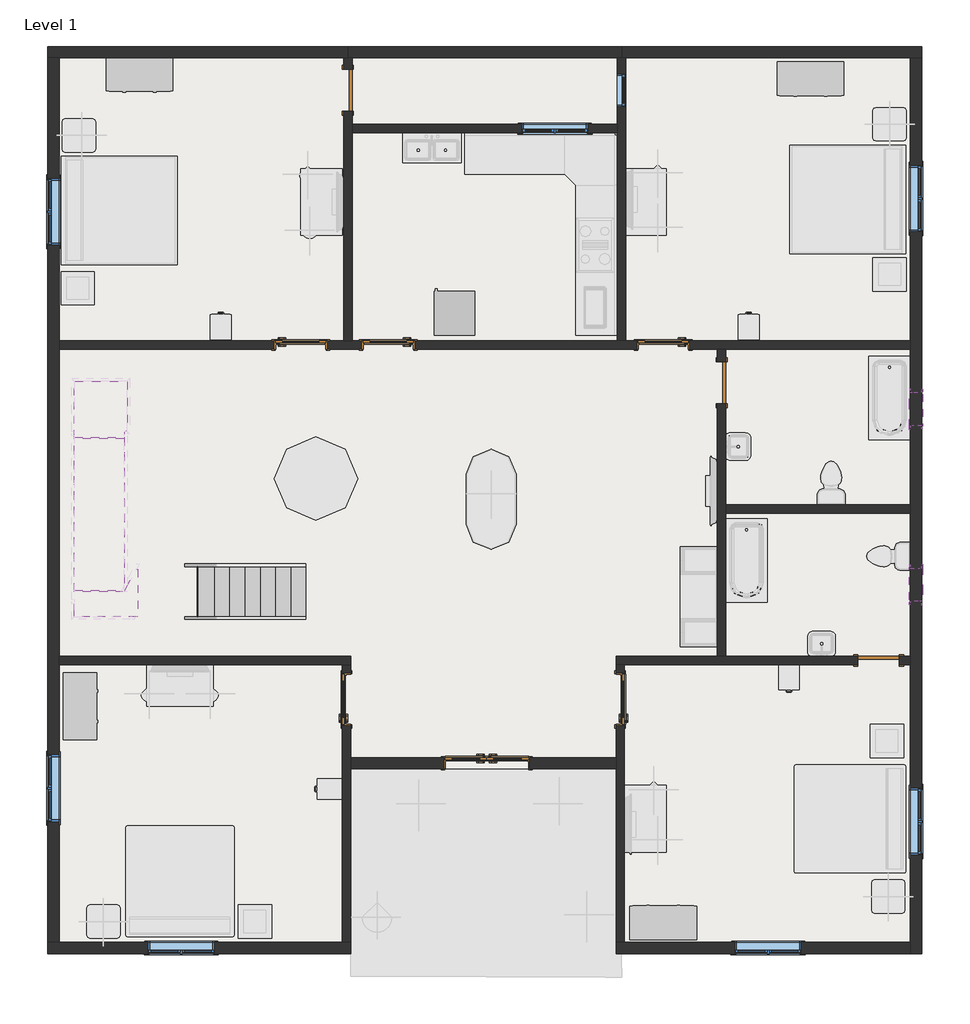
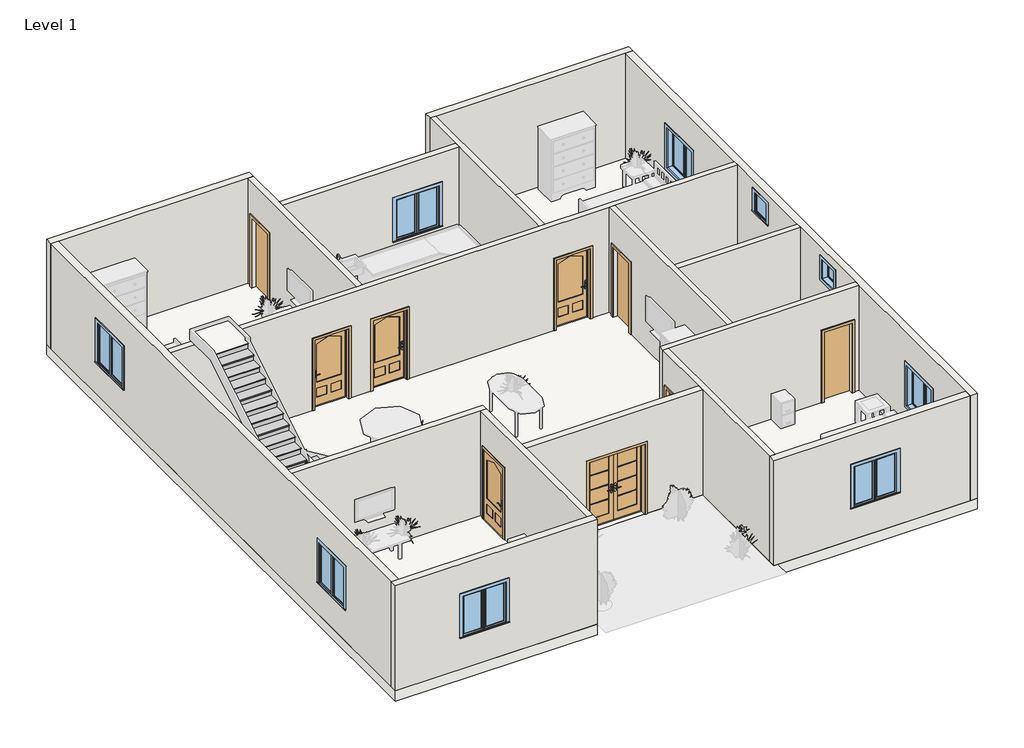
# One storey, part 1 of 2: 18 walls, 10 windows, 9 doors, 3 slabs, 2 stair flights.
"""IFC4 building model written with IfcOpenShell, lengths in millimetres."""

from ifc_helpers import new_model, si_unit, frame, origin, origin_with_axes, place, context, project, spatial, polyline, outline, extrude, faceted_brep, transform, mapped, element, save
from components import door_5d363d20, door_808aeb8e, door_b03bd389, door_059fdd7e, door_255cab33, non_monolithic_landing_7e22f3b9, non_monolithic_landing_d7f15ac0, stair_flight_13c2be00, stair_flight_cee2f43a, window_0862ab64, window_be30da88, window_aff1bc2a, window_e41d21a6

model = new_model("IFC4")

# Units and contexts
model_context = context("Model", 3, world=origin())
ifc_project = project(units=[si_unit("LENGTHUNIT", "METRE", prefix="MILLI")], contexts=[model_context])

# Site, building, storey
site = spatial("IfcSite", under=ifc_project)
building = spatial("IfcBuilding", under=site)
storey = spatial("IfcBuildingStorey", under=building, Name="Level 1", Elevation=0.0)

# Doors
placement = place(None, origin())
door_shape = door_5d363d20(model_context)
element("IfcDoor", 1, ObjectType="36\" x 80\"", at=placement, inside=storey, context=model_context, shape_type="MappedRepresentation", body=[
    mapped(door_shape, transform((-10796.38283, 9355.0370171, 0.0), x_axis=(-1.0, 0.0, 0.0), y_axis=(0.0, -1.0, 0.0), z_axis=(0.0, 0.0, 1.0))),
])
element("IfcDoor", 2, ObjectType="36\" x 80\"", at=placement, inside=storey, context=model_context, shape_type="MappedRepresentation", body=[
    mapped(door_shape, transform((-9961.35783, 2874.8620171, 0.0), x_axis=(0.0, -1.0, 0.0), y_axis=(1.0, 0.0, 0.0), z_axis=(0.0, 0.0, 1.0))),
])
door_2_shape = door_808aeb8e(model_context)
element("IfcDoor", 3, ObjectType="36\" x 80\"", at=placement, inside=storey, context=model_context, shape_type="MappedRepresentation", body=[
    mapped(door_2_shape, transform((-9196.18283, 9355.0370171, 0.0), x_axis=(1.0, 0.0, 0.0), y_axis=(0.0, 1.0, 0.0), z_axis=(0.0, 0.0, 1.0))),
])
element("IfcDoor", 4, ObjectType="36\" x 80\"", at=placement, inside=storey, context=model_context, shape_type="MappedRepresentation", body=[
    mapped(door_2_shape, transform((-4166.98283, 9355.0370171, 0.0), x_axis=(1.0, 0.0, 0.0), y_axis=(0.0, 1.0, 0.0), z_axis=(0.0, 0.0, 1.0))),
])
element("IfcDoor", 5, ObjectType="36\" x 80\"", at=placement, inside=storey, context=model_context, shape_type="MappedRepresentation", body=[
    mapped(door_2_shape, transform((-4951.20783, 2874.8620171, 0.0), x_axis=(0.0, -1.0, 0.0), y_axis=(1.0, 0.0, 0.0), z_axis=(0.0, 0.0, 1.0))),
])
door_3_shape = door_b03bd389(model_context)
element("IfcDoor", 6, ObjectType="Door-Exterior-Double-Full Glass-Wood_Clad : 60\" x 80\"", at=placement, inside=storey, context=model_context, shape_type="MappedRepresentation", body=[
    mapped(door_3_shape, transform((-7392.78283, 1709.6370171, 0.0), x_axis=(1.0, 0.0, 0.0), y_axis=(0.0, 1.0, 0.0), z_axis=(0.0, 0.0, 1.0))),
])
door_4_shape = door_059fdd7e(model_context)
element("IfcDoor", 7, ObjectType="Single-Flush : 30\" x 80\"", at=placement, inside=storey, context=model_context, shape_type="MappedRepresentation", body=[
    mapped(door_4_shape, transform((-229.98283, 3586.0620171, 0.0), x_axis=(1.0, 0.0, 0.0), y_axis=(0.0, 1.0, 0.0), z_axis=(0.0, 0.0, 1.0))),
])
element("IfcDoor", 8, ObjectType="Single-Flush : 30\" x 80\"", at=placement, inside=storey, context=model_context, shape_type="MappedRepresentation", body=[
    mapped(door_4_shape, transform((-9932.78283, 14012.7620171, 0.0), x_axis=(0.0, -1.0, 0.0), y_axis=(1.0, 0.0, 0.0), z_axis=(0.0, 0.0, 1.0))),
])
door_5_shape = door_255cab33(model_context)
element("IfcDoor", 9, ObjectType="Single-Flush : 30\" x 80\"", at=placement, inside=storey, context=model_context, shape_type="MappedRepresentation", body=[
    mapped(door_5_shape, transform((-3100.18283, 8666.0620171, 0.0), x_axis=(0.0, 1.0, 0.0), y_axis=(-1.0, 0.0, 0.0), z_axis=(0.0, 0.0, 1.0))),
])

# Slabs
element("IfcSlab", 10, ObjectType="Generic - 12\"", at=placement, inside=storey, context=model_context, shape_type="SweptSolid", body=[
    extrude(outline(polyline([(557.41717, 14812.8620171), (557.41717, -1773.3379829), (-5030.58283, -1773.3379829), (-5030.58283, 1604.8620171), (-9881.98283, 1604.8620171), (-9881.98283, -1773.3379829), (-15419.18283, -1773.3379829), (-15419.18283, 14812.8620171), (557.41717, 14812.8620171)])), frame((0.0, 0.0, -304.8), z_axis=(0.0, 0.0, 1.0), x_axis=(1.0, 0.0, 0.0)), (0.0, 0.0, 1.0), 304.8),
])
non_monolithic_landing_shape = non_monolithic_landing_7e22f3b9(model_context)
element("IfcSlab", 11, ObjectType="Non-Monolithic Landing", at=placement, inside=storey, context=model_context, shape_type="MappedRepresentation", body=[
    mapped(non_monolithic_landing_shape, transform((0.0, 0.0, 0.0), x_axis=(1.0, 0.0, 0.0), y_axis=(0.0, 1.0, 0.0), z_axis=(0.0, 0.0, 1.0))),
])
non_monolithic_landing_2_shape = non_monolithic_landing_d7f15ac0(model_context)
element("IfcSlab", 12, ObjectType="Non-Monolithic Landing", at=placement, inside=storey, context=model_context, shape_type="MappedRepresentation", body=[
    mapped(non_monolithic_landing_2_shape, transform((0.0, 0.0, 0.0), x_axis=(1.0, 0.0, 0.0), y_axis=(0.0, 1.0, 0.0), z_axis=(0.0, 0.0, 1.0))),
])

# Stair flights
stair_flight_shape = stair_flight_13c2be00(model_context)
element("IfcStairFlight", 13, ObjectType="2\" Tread 1\" Nosing 1/4\" Riser", at=placement, inside=storey, context=model_context, shape_type="MappedRepresentation", body=[
    mapped(stair_flight_shape, transform((0.0, 0.0, 0.0), x_axis=(1.0, 0.0, 0.0), y_axis=(0.0, 1.0, 0.0), z_axis=(0.0, 0.0, 1.0))),
])
stair_flight_2_shape = stair_flight_cee2f43a(model_context)
element("IfcStairFlight", 14, ObjectType="2\" Tread 1\" Nosing 1/4\" Riser", at=placement, inside=storey, context=model_context, shape_type="MappedRepresentation", body=[
    mapped(stair_flight_2_shape, transform((0.0, 0.0, 0.0), x_axis=(1.0, 0.0, 0.0), y_axis=(0.0, 1.0, 0.0), z_axis=(0.0, 0.0, 1.0))),
])

# Walls
element("IfcWall", 15, ObjectType="Generic - 8\"", at=placement, inside=storey, context=model_context, shape_type="Brep", body=[
    faceted_brep([(-15419.18283, 14609.6620171, 0.0), (-15215.98283, 14609.6620171, 0.0), (-10008.98283, 14609.6620171, 0.0), (-9932.78283, 14609.6620171, 0.0), (-9932.78283, 14609.6620171, 1828.8), (-9856.58283, 14609.6620171, 1828.8), (-9856.58283, 14609.6620171, 3048.0), (-10008.98283, 14609.6620171, 3048.0), (-15215.98283, 14609.6620171, 3048.0), (-15419.18283, 14609.6620171, 3048.0), (-15419.18283, 14812.8620171, 0.0), (-15419.18283, 14812.8620171, 3048.0), (-9856.58283, 14812.8620171, 3048.0), (-9856.58283, 14812.8620171, 1828.8), (-9932.78283, 14812.8620171, 1828.8), (-9932.78283, 14812.8620171, 0.0)], [[[0, 1, 2, 3, 4, 5, 6, 7, 8, 9]], [[10, 11, 12, 13, 14, 15]], [[3, 2, 1, 0, 10, 15]], [[0, 9, 11, 10]], [[4, 3, 15, 14]], [[13, 5, 4, 14]], [[6, 5, 13, 12]], [[9, 8, 7, 6, 12, 11]]]),
])
element("IfcWall", 16, ObjectType="Generic - 8\"", at=placement, inside=storey, context=model_context, shape_type="Brep", body=[
    faceted_brep([(354.21717, 14609.6620171, 0.0), (354.21717, 9428.0620171, 0.0), (354.21717, 9275.6620171, 0.0), (354.21717, 6430.8620171, 0.0), (354.21717, 6278.4620171, 0.0), (354.21717, 3662.2620171, 0.0), (354.21717, 3509.8620171, 0.0), (354.21717, -1570.1379829, 0.0), (354.21717, -1773.3379829, 0.0), (354.21717, -1773.3379829, 3048.0), (354.21717, -1570.1379829, 3048.0), (354.21717, 3509.8620171, 3048.0), (354.21717, 3662.2620171, 3048.0), (354.21717, 6278.4620171, 3048.0), (354.21717, 6430.8620171, 3048.0), (354.21717, 9275.6620171, 3048.0), (354.21717, 9428.0620171, 3048.0), (354.21717, 14609.6620171, 3048.0), (354.21717, 11421.9620171, 2133.6), (354.21717, 11421.9620171, 914.4), (354.21717, 12641.1620171, 914.4), (354.21717, 12641.1620171, 2133.6), (354.21717, 30.0620171, 2133.6), (354.21717, 30.0620171, 914.4), (354.21717, 1249.2620171, 914.4), (354.21717, 1249.2620171, 2133.6), (354.21717, 4665.5620171, 2768.6), (354.21717, 4665.5620171, 2159.0), (354.21717, 5275.1620171, 2159.0), (354.21717, 5275.1620171, 2768.6), (354.21717, 8488.2620171, 2768.6), (354.21717, 7878.6620171, 2768.6), (354.21717, 7878.6620171, 2159.0), (354.21717, 8488.2620171, 2159.0), (557.41717, 14609.6620171, 0.0), (557.41717, 14609.6620171, 3048.0), (557.41717, -1773.3379829, 3048.0), (557.41717, -1773.3379829, 0.0), (557.41717, 11421.9620171, 2133.6), (557.41717, 12641.1620171, 2133.6), (557.41717, 12641.1620171, 914.4), (557.41717, 11421.9620171, 914.4), (557.41717, 30.0620171, 2133.6), (557.41717, 1249.2620171, 2133.6), (557.41717, 1249.2620171, 914.4), (557.41717, 30.0620171, 914.4), (557.41717, 4665.5620171, 2768.6), (557.41717, 5275.1620171, 2768.6), (557.41717, 5275.1620171, 2159.0), (557.41717, 4665.5620171, 2159.0), (557.41717, 8488.2620171, 2768.6), (557.41717, 8488.2620171, 2159.0), (557.41717, 7878.6620171, 2159.0), (557.41717, 7878.6620171, 2768.6)], [[[0, 1, 2, 3, 4, 5, 6, 7, 8, 9, 10, 11, 12, 13, 14, 15, 16, 17], [18, 19, 20, 21], [22, 23, 24, 25], [26, 27, 28, 29], [30, 31, 32, 33]], [[34, 35, 36, 37], [38, 39, 40, 41], [42, 43, 44, 45], [46, 47, 48, 49], [50, 51, 52, 53]], [[8, 7, 6, 5, 4, 3, 2, 1, 0, 34, 37]], [[0, 17, 35, 34]], [[9, 8, 37, 36]], [[19, 18, 38, 41]], [[20, 19, 41, 40]], [[21, 20, 40, 39]], [[18, 21, 39, 38]], [[23, 22, 42, 45]], [[24, 23, 45, 44]], [[25, 24, 44, 43]], [[22, 25, 43, 42]], [[27, 26, 46, 49]], [[28, 27, 49, 48]], [[29, 28, 48, 47]], [[26, 29, 47, 46]], [[51, 50, 30, 33]], [[52, 51, 33, 32]], [[53, 52, 32, 31]], [[50, 53, 31, 30]], [[17, 16, 15, 14, 13, 12, 11, 10, 9, 36, 35]]]),
])
element("IfcWall", 17, ObjectType="Generic - 8\"", at=placement, inside=storey, context=model_context, shape_type="Brep", body=[
    faceted_brep([(354.21717, -1570.1379829, 0.0), (-4878.18283, -1570.1379829, 0.0), (-5030.58283, -1570.1379829, 0.0), (-5030.58283, -1570.1379829, 3048.0), (-4878.18283, -1570.1379829, 3048.0), (354.21717, -1570.1379829, 3048.0), (-2858.88283, -1570.1379829, 2133.6), (-2858.88283, -1570.1379829, 914.4), (-1639.68283, -1570.1379829, 914.4), (-1639.68283, -1570.1379829, 2133.6), (354.21717, -1773.3379829, 0.0), (354.21717, -1773.3379829, 3048.0), (-5030.58283, -1773.3379829, 3048.0), (-5030.58283, -1773.3379829, 0.0), (-2858.88283, -1773.3379829, 2133.6), (-1639.68283, -1773.3379829, 2133.6), (-1639.68283, -1773.3379829, 914.4), (-2858.88283, -1773.3379829, 914.4)], [[[0, 1, 2, 3, 4, 5], [6, 7, 8, 9]], [[10, 11, 12, 13], [14, 15, 16, 17]], [[2, 1, 0, 10, 13]], [[0, 5, 11, 10]], [[3, 2, 13, 12]], [[7, 6, 14, 17]], [[8, 7, 17, 16]], [[9, 8, 16, 15]], [[6, 9, 15, 14]], [[5, 4, 3, 12, 11]]]),
])
element("IfcWall", 18, ObjectType="Generic - 8\"", at=placement, inside=storey, context=model_context, shape_type="Brep", body=[
    faceted_brep([(-15215.98283, -1570.1379829, 0.0), (-15215.98283, 3509.8620171, 0.0), (-15215.98283, 3662.2620171, 0.0), (-15215.98283, 9275.6620171, 0.0), (-15215.98283, 9428.0620171, 0.0), (-15215.98283, 14609.6620171, 0.0), (-15215.98283, 14609.6620171, 3048.0), (-15215.98283, 9428.0620171, 3048.0), (-15215.98283, 9275.6620171, 3048.0), (-15215.98283, 3662.2620171, 3048.0), (-15215.98283, 3509.8620171, 3048.0), (-15215.98283, -1570.1379829, 3048.0), (-15215.98283, 12399.8620171, 2133.6), (-15215.98283, 12399.8620171, 914.4), (-15215.98283, 11180.6620171, 914.4), (-15215.98283, 11180.6620171, 2133.6), (-15215.98283, 1858.8620171, 2133.6), (-15215.98283, 1858.8620171, 914.4), (-15215.98283, 639.6620171, 914.4), (-15215.98283, 639.6620171, 2133.6), (-15419.18283, -1570.1379829, 0.0), (-15419.18283, -1570.1379829, 3048.0), (-15419.18283, 14609.6620171, 3048.0), (-15419.18283, 14609.6620171, 0.0), (-15419.18283, 12399.8620171, 2133.6), (-15419.18283, 11180.6620171, 2133.6), (-15419.18283, 11180.6620171, 914.4), (-15419.18283, 12399.8620171, 914.4), (-15419.18283, 1858.8620171, 2133.6), (-15419.18283, 639.6620171, 2133.6), (-15419.18283, 639.6620171, 914.4), (-15419.18283, 1858.8620171, 914.4)], [[[0, 1, 2, 3, 4, 5, 6, 7, 8, 9, 10, 11], [12, 13, 14, 15], [16, 17, 18, 19]], [[20, 21, 22, 23], [24, 25, 26, 27], [28, 29, 30, 31]], [[5, 4, 3, 2, 1, 0, 20, 23]], [[6, 5, 23, 22]], [[0, 11, 21, 20]], [[13, 12, 24, 27]], [[14, 13, 27, 26]], [[15, 14, 26, 25]], [[12, 15, 25, 24]], [[17, 16, 28, 31]], [[18, 17, 31, 30]], [[19, 18, 30, 29]], [[16, 19, 29, 28]], [[11, 10, 9, 8, 7, 6, 22, 21]]]),
])
element("IfcWall", 19, ObjectType="Generic - 8\"", at=placement, inside=storey, context=model_context, shape_type="SweptSolid", body=[
    extrude(outline(polyline([(3048.0, -9881.98283), (0.0, -9881.98283), (0.0, -8180.18283), (2057.4, -8180.18283), (2057.4, -6605.38283), (0.0, -6605.38283), (0.0, -5030.58283), (3048.0, -5030.58283), (3048.0, -9881.98283)])), frame((0.0, 1604.8620171, 0.0), z_axis=(0.0, 1.0, 0.0), x_axis=(0.0, 0.0, 1.0)), (0.0, 0.0, 1.0), 203.2),
])
element("IfcWall", 20, ObjectType="Generic - 8\"", at=placement, inside=storey, context=model_context, shape_type="Brep", body=[
    faceted_brep([(-9881.98283, -1570.1379829, 0.0), (-10034.38283, -1570.1379829, 0.0), (-15215.98283, -1570.1379829, 0.0), (-15419.18283, -1570.1379829, 0.0), (-15419.18283, -1570.1379829, 3048.0), (-15215.98283, -1570.1379829, 3048.0), (-10034.38283, -1570.1379829, 3048.0), (-9881.98283, -1570.1379829, 3048.0), (-13590.38283, -1570.1379829, 2133.6), (-13590.38283, -1570.1379829, 914.4), (-12371.18283, -1570.1379829, 914.4), (-12371.18283, -1570.1379829, 2133.6), (-9881.98283, -1773.3379829, 0.0), (-9881.98283, -1773.3379829, 3048.0), (-15419.18283, -1773.3379829, 3048.0), (-15419.18283, -1773.3379829, 0.0), (-13590.38283, -1773.3379829, 2133.6), (-12371.18283, -1773.3379829, 2133.6), (-12371.18283, -1773.3379829, 914.4), (-13590.38283, -1773.3379829, 914.4)], [[[0, 1, 2, 3, 4, 5, 6, 7], [8, 9, 10, 11]], [[12, 13, 14, 15], [16, 17, 18, 19]], [[3, 2, 1, 0, 12, 15]], [[4, 3, 15, 14]], [[0, 7, 13, 12]], [[9, 8, 16, 19]], [[10, 9, 19, 18]], [[11, 10, 18, 17]], [[8, 11, 17, 16]], [[7, 6, 5, 4, 14, 13]]]),
])
element("IfcWall", 21, ObjectType="Generic - 8\"", at=placement, inside=storey, context=model_context, shape_type="Brep", body=[
    faceted_brep([(-4928.98283, 14609.6620171, 0.0), (-4852.78283, 14609.6620171, 0.0), (354.21717, 14609.6620171, 0.0), (557.41717, 14609.6620171, 0.0), (557.41717, 14609.6620171, 3048.0), (354.21717, 14609.6620171, 3048.0), (-4852.78283, 14609.6620171, 3048.0), (-5005.18283, 14609.6620171, 3048.0), (-5005.18283, 14609.6620171, 1828.8), (-4928.98283, 14609.6620171, 1828.8), (-4928.98283, 14812.8620171, 0.0), (-4928.98283, 14812.8620171, 1828.8), (-5005.18283, 14812.8620171, 1828.8), (-5005.18283, 14812.8620171, 3048.0), (557.41717, 14812.8620171, 3048.0), (557.41717, 14812.8620171, 0.0)], [[[0, 1, 2, 3, 4, 5, 6, 7, 8, 9]], [[10, 11, 12, 13, 14, 15]], [[3, 2, 1, 0, 10, 15]], [[4, 3, 15, 14]], [[0, 9, 11, 10]], [[8, 12, 11, 9]], [[8, 7, 13, 12]], [[7, 6, 5, 4, 14, 13]]]),
])
element("IfcWall", 22, ObjectType="Generic - 8\"", at=placement, inside=storey, context=model_context, shape_type="Brep", body=[
    faceted_brep([(-9932.78283, 14609.6620171, 0.0), (-9856.58283, 14609.6620171, 0.0), (-5005.18283, 14609.6620171, 0.0), (-4928.98283, 14609.6620171, 0.0), (-4928.98283, 14609.6620171, 1828.8), (-5005.18283, 14609.6620171, 1828.8), (-9856.58283, 14609.6620171, 1828.8), (-9932.78283, 14609.6620171, 1828.8), (-9932.78283, 14812.8620171, 0.0), (-9932.78283, 14812.8620171, 1828.8), (-9856.58283, 14812.8620171, 1828.8), (-5005.18283, 14812.8620171, 1828.8), (-4928.98283, 14812.8620171, 1828.8), (-4928.98283, 14812.8620171, 0.0)], [[[0, 1, 2, 3, 4, 5, 6, 7]], [[8, 9, 10, 11, 12, 13]], [[3, 2, 1, 0, 8, 13]], [[4, 3, 13, 12]], [[7, 6, 5, 4, 12, 11, 10, 9]], [[0, 7, 9, 8]]]),
])
element("IfcWall", 23, ObjectType="INNER 6\"", at=placement, inside=storey, context=model_context, shape_type="Brep", body=[
    faceted_brep([(-10008.98283, 13631.7620171, 2032.0), (-10008.98283, 13631.7620171, 0.0), (-10008.98283, 9428.0620171, 0.0), (-10008.98283, 9428.0620171, 3048.0), (-10008.98283, 14609.6620171, 3048.0), (-10008.98283, 14609.6620171, 0.0), (-10008.98283, 14393.7620171, 0.0), (-10008.98283, 14393.7620171, 2032.0), (-9856.58283, 9428.0620171, 0.0), (-9856.58283, 13238.0620171, 0.0), (-9856.58283, 13390.4620171, 0.0), (-9856.58283, 13631.7620171, 0.0), (-9856.58283, 13631.7620171, 2032.0), (-9856.58283, 14393.7620171, 2032.0), (-9856.58283, 14393.7620171, 0.0), (-9856.58283, 14609.6620171, 0.0), (-9856.58283, 14609.6620171, 1828.8), (-9856.58283, 14609.6620171, 3048.0), (-9856.58283, 13390.4620171, 3048.0), (-9856.58283, 13238.0620171, 3048.0), (-9856.58283, 9428.0620171, 3048.0), (-9932.78283, 14609.6620171, 0.0)], [[[0, 1, 2, 3, 4, 5, 6, 7]], [[8, 9, 10, 11, 12, 13, 14, 15, 16, 17, 18, 19, 20]], [[6, 5, 21, 15, 14]], [[2, 1, 11, 10, 9, 8]], [[3, 2, 8, 20]], [[12, 11, 1, 0]], [[13, 12, 0, 7]], [[14, 13, 7, 6]], [[4, 17, 16, 15, 21, 5]], [[4, 3, 20, 19, 18, 17]]]),
])
element("IfcWall", 24, ObjectType="INNER 6\"", at=placement, inside=storey, context=model_context, shape_type="Brep", body=[
    faceted_brep([(-15215.98283, 9428.0620171, 0.0), (-15215.98283, 9428.0620171, 3048.0), (-10008.98283, 9428.0620171, 3048.0), (-9856.58283, 9428.0620171, 3048.0), (-5005.18283, 9428.0620171, 3048.0), (-4852.78283, 9428.0620171, 3048.0), (354.21717, 9428.0620171, 3048.0), (354.21717, 9428.0620171, 0.0), (-3684.38283, 9428.0620171, 0.0), (-3684.38283, 9428.0620171, 2057.4), (-4649.58283, 9428.0620171, 2057.4), (-4649.58283, 9428.0620171, 0.0), (-4852.78283, 9428.0620171, 0.0), (-5005.18283, 9428.0620171, 0.0), (-8713.58283, 9428.0620171, 0.0), (-8713.58283, 9428.0620171, 2057.4), (-9678.78283, 9428.0620171, 2057.4), (-9678.78283, 9428.0620171, 0.0), (-9856.58283, 9428.0620171, 0.0), (-10008.98283, 9428.0620171, 0.0), (-10313.78283, 9428.0620171, 0.0), (-10313.78283, 9428.0620171, 2057.4), (-11278.98283, 9428.0620171, 2057.4), (-11278.98283, 9428.0620171, 0.0), (-15215.98283, 9275.6620171, 3048.0), (-15215.98283, 9275.6620171, 0.0), (-11278.98283, 9275.6620171, 0.0), (-11278.98283, 9275.6620171, 2057.4), (-10313.78283, 9275.6620171, 2057.4), (-10313.78283, 9275.6620171, 0.0), (-9678.78283, 9275.6620171, 0.0), (-9678.78283, 9275.6620171, 2057.4), (-8713.58283, 9275.6620171, 2057.4), (-8713.58283, 9275.6620171, 0.0), (-4649.58283, 9275.6620171, 0.0), (-4649.58283, 9275.6620171, 2057.4), (-3684.38283, 9275.6620171, 2057.4), (-3684.38283, 9275.6620171, 0.0), (-3176.38283, 9275.6620171, 0.0), (-3023.98283, 9275.6620171, 0.0), (354.21717, 9275.6620171, 0.0), (354.21717, 9275.6620171, 3048.0), (-3023.98283, 9275.6620171, 3048.0), (-3176.38283, 9275.6620171, 3048.0)], [[[0, 1, 2, 3, 4, 5, 6, 7, 8, 9, 10, 11, 12, 13, 14, 15, 16, 17, 18, 19, 20, 21, 22, 23]], [[24, 25, 26, 27, 28, 29, 30, 31, 32, 33, 34, 35, 36, 37, 38, 39, 40, 41, 42, 43]], [[25, 0, 23, 26]], [[7, 40, 39, 38, 37, 8]], [[29, 20, 19, 18, 17, 30]], [[33, 14, 13, 12, 11, 34]], [[1, 0, 25, 24]], [[7, 6, 41, 40]], [[22, 27, 26, 23]], [[27, 22, 21, 28]], [[28, 21, 20, 29]], [[32, 15, 14, 33]], [[15, 32, 31, 16]], [[16, 31, 30, 17]], [[36, 9, 8, 37]], [[9, 36, 35, 10]], [[10, 35, 34, 11]], [[6, 5, 4, 3, 2, 1, 24, 43, 42, 41]]]),
])
element("IfcWall", 25, ObjectType="INNER 6\"", at=placement, inside=storey, context=model_context, shape_type="Brep", body=[
    faceted_brep([(-5005.18283, 14609.6620171, 3048.0), (-5005.18283, 14609.6620171, 1828.8), (-5005.18283, 14609.6620171, 0.0), (-5005.18283, 13390.4620171, 0.0), (-5005.18283, 13238.0620171, 0.0), (-5005.18283, 9428.0620171, 0.0), (-5005.18283, 9428.0620171, 3048.0), (-5005.18283, 13238.0620171, 3048.0), (-5005.18283, 13390.4620171, 3048.0), (-5005.18283, 13707.9620171, 1524.0), (-5005.18283, 13707.9620171, 914.4), (-5005.18283, 14317.5620171, 914.4), (-5005.18283, 14317.5620171, 1524.0), (-4852.78283, 14609.6620171, 0.0), (-4852.78283, 14609.6620171, 3048.0), (-4852.78283, 9428.0620171, 3048.0), (-4852.78283, 9428.0620171, 0.0), (-4852.78283, 13707.9620171, 1524.0), (-4852.78283, 14317.5620171, 1524.0), (-4852.78283, 14317.5620171, 914.4), (-4852.78283, 13707.9620171, 914.4), (-4928.98283, 14609.6620171, 0.0)], [[[0, 1, 2, 3, 4, 5, 6, 7, 8], [9, 10, 11, 12]], [[13, 14, 15, 16], [17, 18, 19, 20]], [[5, 4, 3, 2, 21, 13, 16]], [[6, 5, 16, 15]], [[10, 9, 17, 20]], [[11, 10, 20, 19]], [[12, 11, 19, 18]], [[9, 12, 18, 17]], [[0, 14, 13, 21, 2, 1]], [[0, 8, 7, 6, 15, 14]]]),
])
element("IfcWall", 26, ObjectType="INNER 6\"", at=placement, inside=storey, context=model_context, shape_type="SweptSolid", body=[
    extrude(outline(polyline([(0.0, -5005.18283), (3048.0, -5005.18283), (3048.0, -9856.58283), (0.0, -9856.58283), (0.0, -5005.18283)]), holes=[polyline([(2133.6, -6757.78283), (2133.6, -5538.58283), (914.4, -5538.58283), (914.4, -6757.78283), (2133.6, -6757.78283)])]), frame((0.0, 13238.0620171, 0.0), z_axis=(0.0, 1.0, 0.0), x_axis=(0.0, 0.0, 1.0)), (0.0, 0.0, 1.0), 152.4),
])
element("IfcWall", 27, ObjectType="INNER 6\"", at=placement, inside=storey, context=model_context, shape_type="Brep", body=[
    faceted_brep([(-15215.98283, 3509.8620171, 0.0), (-10034.38283, 3509.8620171, 0.0), (-9881.98283, 3509.8620171, 0.0), (-9881.98283, 3509.8620171, 3048.0), (-10034.38283, 3509.8620171, 3048.0), (-15215.98283, 3509.8620171, 3048.0), (-15215.98283, 3662.2620171, 0.0), (-15215.98283, 3662.2620171, 3048.0), (-9881.98283, 3662.2620171, 3048.0), (-9881.98283, 3662.2620171, 0.0)], [[[0, 1, 2, 3, 4, 5]], [[6, 7, 8, 9]], [[2, 1, 0, 6, 9]], [[0, 5, 7, 6]], [[3, 2, 9, 8]], [[5, 4, 3, 8, 7]]]),
])
element("IfcWall", 28, ObjectType="INNER 6\"", at=placement, inside=storey, context=model_context, shape_type="Brep", body=[
    faceted_brep([(-10034.38283, 3509.8620171, 3048.0), (-10034.38283, 3509.8620171, 0.0), (-10034.38283, 3357.4620171, 0.0), (-10034.38283, 3357.4620171, 2057.4), (-10034.38283, 2392.2620171, 2057.4), (-10034.38283, 2392.2620171, 0.0), (-10034.38283, -1570.1379829, 0.0), (-10034.38283, -1570.1379829, 3048.0), (-9881.98283, 3509.8620171, 0.0), (-9881.98283, 3509.8620171, 3048.0), (-9881.98283, 1808.0620171, 3048.0), (-9881.98283, 1604.8620171, 3048.0), (-9881.98283, -1570.1379829, 3048.0), (-9881.98283, -1570.1379829, 0.0), (-9881.98283, 1604.8620171, 0.0), (-9881.98283, 1808.0620171, 0.0), (-9881.98283, 2392.2620171, 0.0), (-9881.98283, 2392.2620171, 2057.4), (-9881.98283, 3357.4620171, 2057.4), (-9881.98283, 3357.4620171, 0.0)], [[[0, 1, 2, 3, 4, 5, 6, 7]], [[8, 9, 10, 11, 12, 13, 14, 15, 16, 17, 18, 19]], [[1, 8, 19, 2]], [[13, 6, 5, 16, 15, 14]], [[1, 0, 9, 8]], [[7, 6, 13, 12]], [[4, 17, 16, 5]], [[17, 4, 3, 18]], [[18, 3, 2, 19]], [[0, 7, 12, 11, 10, 9]]]),
])
element("IfcWall", 29, ObjectType="INNER 6\"", at=placement, inside=storey, context=model_context, shape_type="Brep", body=[
    faceted_brep([(354.21717, 3662.2620171, 0.0), (151.01717, 3662.2620171, 0.0), (151.01717, 3662.2620171, 2032.0), (-610.98283, 3662.2620171, 2032.0), (-610.98283, 3662.2620171, 0.0), (-3023.98283, 3662.2620171, 0.0), (-3176.38283, 3662.2620171, 0.0), (-5030.58283, 3662.2620171, 0.0), (-5030.58283, 3662.2620171, 3048.0), (-3176.38283, 3662.2620171, 3048.0), (-3023.98283, 3662.2620171, 3048.0), (354.21717, 3662.2620171, 3048.0), (151.01717, 3509.8620171, 2032.0), (151.01717, 3509.8620171, 0.0), (354.21717, 3509.8620171, 0.0), (354.21717, 3509.8620171, 3048.0), (-4878.18283, 3509.8620171, 3048.0), (-5030.58283, 3509.8620171, 3048.0), (-5030.58283, 3509.8620171, 0.0), (-4878.18283, 3509.8620171, 0.0), (-610.98283, 3509.8620171, 0.0), (-610.98283, 3509.8620171, 2032.0)], [[[0, 1, 2, 3, 4, 5, 6, 7, 8, 9, 10, 11]], [[12, 13, 14, 15, 16, 17, 18, 19, 20, 21]], [[14, 13, 1, 0]], [[20, 19, 18, 7, 6, 5, 4]], [[0, 11, 15, 14]], [[8, 7, 18, 17]], [[2, 1, 13, 12]], [[3, 2, 12, 21]], [[4, 3, 21, 20]], [[11, 10, 9, 8, 17, 16, 15]]]),
])
element("IfcWall", 30, ObjectType="INNER 6\"", at=placement, inside=storey, context=model_context, shape_type="Brep", body=[
    faceted_brep([(-5030.58283, 3509.8620171, 3048.0), (-5030.58283, 3509.8620171, 0.0), (-5030.58283, 3357.4620171, 0.0), (-5030.58283, 3357.4620171, 2057.4), (-5030.58283, 2392.2620171, 2057.4), (-5030.58283, 2392.2620171, 0.0), (-5030.58283, 1808.0620171, 0.0), (-5030.58283, 1604.8620171, 0.0), (-5030.58283, -1570.1379829, 0.0), (-5030.58283, -1570.1379829, 3048.0), (-5030.58283, 1604.8620171, 3048.0), (-5030.58283, 1808.0620171, 3048.0), (-4878.18283, 3509.8620171, 0.0), (-4878.18283, 3509.8620171, 3048.0), (-4878.18283, -1570.1379829, 3048.0), (-4878.18283, -1570.1379829, 0.0), (-4878.18283, 2392.2620171, 0.0), (-4878.18283, 2392.2620171, 2057.4), (-4878.18283, 3357.4620171, 2057.4), (-4878.18283, 3357.4620171, 0.0)], [[[0, 1, 2, 3, 4, 5, 6, 7, 8, 9, 10, 11]], [[12, 13, 14, 15, 16, 17, 18, 19]], [[1, 12, 19, 2]], [[15, 8, 7, 6, 5, 16]], [[1, 0, 13, 12]], [[9, 8, 15, 14]], [[4, 17, 16, 5]], [[17, 4, 3, 18]], [[18, 3, 2, 19]], [[0, 11, 10, 9, 14, 13]]]),
])
element("IfcWall", 31, ObjectType="INNER 6\"", at=placement, inside=storey, context=model_context, shape_type="SweptSolid", body=[
    extrude(outline(polyline([(-3023.98283, 6430.8620171), (354.21717, 6430.8620171), (354.21717, 6278.4620171), (-3023.98283, 6278.4620171), (-3023.98283, 6430.8620171)])), origin_with_axes(), (0.0, 0.0, 1.0), 3048.0),
])
element("IfcWall", 32, ObjectType="INNER 6\"", at=placement, inside=storey, context=model_context, shape_type="Brep", body=[
    faceted_brep([(-3176.38283, 9275.6620171, 0.0), (-3176.38283, 9047.0620171, 0.0), (-3176.38283, 9047.0620171, 2032.0), (-3176.38283, 8285.0620171, 2032.0), (-3176.38283, 8285.0620171, 0.0), (-3176.38283, 3662.2620171, 0.0), (-3176.38283, 3662.2620171, 3048.0), (-3176.38283, 9275.6620171, 3048.0), (-3023.98283, 9047.0620171, 2032.0), (-3023.98283, 9047.0620171, 0.0), (-3023.98283, 9275.6620171, 0.0), (-3023.98283, 9275.6620171, 3048.0), (-3023.98283, 6430.8620171, 3048.0), (-3023.98283, 6278.4620171, 3048.0), (-3023.98283, 3662.2620171, 3048.0), (-3023.98283, 3662.2620171, 0.0), (-3023.98283, 6278.4620171, 0.0), (-3023.98283, 6430.8620171, 0.0), (-3023.98283, 8285.0620171, 0.0), (-3023.98283, 8285.0620171, 2032.0)], [[[0, 1, 2, 3, 4, 5, 6, 7]], [[8, 9, 10, 11, 12, 13, 14, 15, 16, 17, 18, 19]], [[10, 9, 1, 0]], [[18, 17, 16, 15, 5, 4]], [[6, 5, 15, 14]], [[0, 7, 11, 10]], [[2, 1, 9, 8]], [[3, 2, 8, 19]], [[4, 3, 19, 18]], [[7, 6, 14, 13, 12, 11]]]),
])

# Windows
window_shape = window_0862ab64(model_context)
element("IfcWindow", 33, ObjectType="Casement Dbl with Trim : 48\" x 48\"", at=placement, inside=storey, context=model_context, shape_type="MappedRepresentation", body=[
    mapped(window_shape, transform((-15298.53283, 11790.2620171, 0.0), x_axis=(0.0, 1.0, 0.0), y_axis=(-1.0, 0.0, 0.0), z_axis=(0.0, 0.0, 1.0))),
])
element("IfcWindow", 34, ObjectType="Casement Dbl with Trim : 48\" x 48\"", at=placement, inside=storey, context=model_context, shape_type="MappedRepresentation", body=[
    mapped(window_shape, transform((436.76717, 12031.5620171, 0.0), x_axis=(0.0, -1.0, 0.0), y_axis=(1.0, 0.0, 0.0), z_axis=(0.0, 0.0, 1.0))),
])
element("IfcWindow", 35, ObjectType="Casement Dbl with Trim : 48\" x 48\"", at=placement, inside=storey, context=model_context, shape_type="MappedRepresentation", body=[
    mapped(window_shape, transform((436.76717, 639.6620171, 0.0), x_axis=(0.0, -1.0, 0.0), y_axis=(1.0, 0.0, 0.0), z_axis=(0.0, 0.0, 1.0))),
])
element("IfcWindow", 36, ObjectType="Casement Dbl with Trim : 48\" x 48\"", at=placement, inside=storey, context=model_context, shape_type="MappedRepresentation", body=[
    mapped(window_shape, transform((-2249.28283, -1652.6879829, 0.0), x_axis=(-1.0, 0.0, 0.0), y_axis=(0.0, -1.0, 0.0), z_axis=(0.0, 0.0, 1.0))),
])
element("IfcWindow", 37, ObjectType="Casement Dbl with Trim : 48\" x 48\"", at=placement, inside=storey, context=model_context, shape_type="MappedRepresentation", body=[
    mapped(window_shape, transform((-12980.78283, -1652.6879829, 0.0), x_axis=(-1.0, 0.0, 0.0), y_axis=(0.0, -1.0, 0.0), z_axis=(0.0, 0.0, 1.0))),
])
element("IfcWindow", 38, ObjectType="Casement Dbl with Trim : 48\" x 48\"", at=placement, inside=storey, context=model_context, shape_type="MappedRepresentation", body=[
    mapped(window_shape, transform((-15298.53283, 1249.2620171, 0.0), x_axis=(0.0, 1.0, 0.0), y_axis=(-1.0, 0.0, 0.0), z_axis=(0.0, 0.0, 1.0))),
])
window_2_shape = window_be30da88(model_context)
element("IfcWindow", 39, ObjectType="Casement Dbl with Trim : 48\" x 48\"", at=placement, inside=storey, context=model_context, shape_type="MappedRepresentation", body=[
    mapped(window_2_shape, transform((-6148.18283, 13333.3120171, 0.0), x_axis=(-1.0, 0.0, 0.0), y_axis=(0.0, -1.0, 0.0), z_axis=(0.0, 0.0, 1.0))),
])
window_3_shape = window_aff1bc2a(model_context)
element("IfcWindow", 40, ObjectType="Fixed : 24\" x 24\"", at=placement, inside=storey, context=model_context, shape_type="MappedRepresentation", body=[
    mapped(window_3_shape, transform((-4928.98283, 13974.6620171, 0.0), x_axis=(0.0, -1.0, 0.0), y_axis=(1.0, 0.0, 0.0), z_axis=(0.0, 0.0, 1.0))),
])
window_4_shape = window_e41d21a6(model_context)
element("IfcWindow", 41, ObjectType="Transom with Trim : 24\" x 24\"", at=placement, inside=storey, context=model_context, shape_type="MappedRepresentation", body=[
    mapped(window_4_shape, transform((455.81717, 4932.2620171, 0.0), x_axis=(0.0, -1.0, 0.0), y_axis=(1.0, 0.0, 0.0), z_axis=(0.0, 0.0, 1.0))),
])
element("IfcWindow", 42, ObjectType="Transom with Trim : 24\" x 24\"", at=placement, inside=storey, context=model_context, shape_type="MappedRepresentation", body=[
    mapped(window_4_shape, transform((455.81717, 8221.5620171, 0.0), x_axis=(0.0, 1.0, 0.0), y_axis=(-1.0, 0.0, 0.0), z_axis=(0.0, 0.0, 1.0))),
])

save(model, "model.ifc")

# Revit data of these elements
# Type "36\" x 80\""
#   Type Mark = "8"
#   Assembly Code = "B2030100"
#   Analytic Construction = "French door, wood frame with single glass"
#   Threshold Offset [instance default] = 0' - 0 1/2"
#   Thickness = 0' - 1 3/8"
#   Thermal Resistance (R) = 1.0696 (h·ft²·°F)/BTU
#   Swing Angle [instance default] = 90.00°
#   Stiles = 0' - 4 3/4"
#   Rough Width = 3' - 2"
#   Rough Height = 6' - 9"
#   Radius = 1' - 8.05625"
#   Lock Rail = 0' - 7 1/8"
#   Height = 6' - 8"
#   Width = 3' - 0"
#   Heat Transfer Coefficient (U) = 0.9350 BTU/(h·ft²·°F)
#   Door Offset [instance default] = 0' - 0"
#   Bottom Rail = 0' - 9 1/2"
#   Threshold [instance default] = yes
#   Function = 1
#   Exterior Trim [instance default] = yes
#   Trim Material = Cherry
#   Threshold Material = Cherry
#   Panel Material = Cherry
#   Glazing = Glass
#   Frame Material = Cherry
#   Door Handle Material = Aluminum
#   Visual Light Transmittance = 0
#   Solar Heat Gain Coefficient = 0
#   Wall Closure = (empty or 0)
#   Construction Type = (empty or 0)
# Type "Door-Exterior-Double-Full Glass-Wood_Clad : 60\" x 80\""
#   Type Mark = "9"
#   Assembly Code = "B2030100"
#   Analytic Construction = "French door, wood frame with double glass"
#   Top Rail = 0' - 4 11/16"
#   Threshold Offset [instance default] = 0' - 0 1/2"
#   Thickness = 0' - 1 3/8"
#   Thermal Resistance (R) = 1.9158 (h·ft²·°F)/BTU
#   Swing Angle [instance default] = 90.00°
#   Stiles = 0' - 4 3/4"
#   Rough Width = 5' - 2"
#   Rough Height = 6' - 9"
#   Panel Width = 2' - 6"
#   Door Offset [instance default] = 0' - 0"
#   Height = 6' - 8"
#   Width = 5' - 0"
#   Heat Transfer Coefficient (U) = 0.5220 BTU/(h·ft²·°F)
#   Bottom Rail = 0' - 9 1/8"
#   Exterior Trim [instance default] = yes
#   Threshold [instance default] = yes
#   Show Grill [instance default] = yes
#   Function = 1
#   Trim Material = Cherry
#   Threshold Material = Cherry
#   Panel Material = Cherry
#   Glazing = Glass
#   Frame Material = Cherry
#   Door Handle Material = Aluminum
#   Visual Light Transmittance = 0
#   Solar Heat Gain Coefficient = 0
#   Wall Closure = (empty or 0)
#   Construction Type = (empty or 0)
# Type "Single-Flush : 30\" x 80\""
#   Type Mark = "5"
#   Construction Type Id = "MDOOR"
#   Assembly Code = "C1020"
#   Analytic Construction = "Metal"
#   Thickness = 0' - 2"
#   Heat Transfer Coefficient (U) = 0.651978 BTU/(h·ft²·°F)
#   Height = 6' - 8"
#   Trim Projection Ext = 0' - 1"
#   Trim Projection Int = 0' - 1"
#   Trim Width = 0' - 3"
#   Width = 2' - 6"
#   Define Thermal Properties by = 1
#   Door Material = Door - Panel
#   Frame Material = Door - Frame
#   Visual Light Transmittance = 0
#   Solar Heat Gain Coefficient = 0
#   Function = (empty or 0)
#   Wall Closure = (empty or 0)
# Type "Generic - 12\""
#   Assembly Code = "B1010"
#   Function = 0
#   Layers, outside or top first: 1' - 0" no material (function 1)
# Type "Generic - 8\""
#   Assembly Code = "B2010"
#   Layers, outside or top first: 0' - 8" "Brick, Common" (function 1)
# Type "INNER 6\""
#   Assembly Code = "B2010"
#   Layers, outside or top first: 0' - 6" "Brick, Common" (function 1)
# Type "Casement Dbl with Trim : 48\" x 48\""
#   Type Mark = "10"
#   Construction Type Id = "GSP4R"
#   Assembly Code = "B2020100"
#   Analytic Construction = "1/8 in Pilkington single glazing"
#   Visual Light Transmittance = 0.9
#   Solar Heat Gain Coefficient = 0.78
#   Heat Transfer Coefficient (U) = 0.6496 BTU/(h·ft²·°F)
#   Height = 4' - 0"
#   Default Sill Height = 3' - 0"
#   Trim Projection - Ext. = 0' - 0 1/2"
#   Trim Projection - Int. = 0' - 0 3/4"
#   Trim Width - Exterior = 0' - 3 1/2"
#   Trim Width - Interior = 0' - 3 1/2"
#   Width = 4' - 0"
#   Window Inset = 0' - 0 3/4"
#   Define Thermal Properties by = 1
#   Glass Pane Material = Glass
#   Sash Material = Sash
#   Trim Exterior Material = Trim
#   Trim Interior Material = Trim
#   Wall Closure = (empty or 0)
# Type "Fixed : 24\" x 24\""
#   Type Mark = "3"
#   Construction Type Id = "GSP4R"
#   Assembly Code = "B2020100"
#   Analytic Construction = "1/8 in Pilkington single glazing"
#   Visual Light Transmittance = 0.9
#   Solar Heat Gain Coefficient = 0.78
#   Heat Transfer Coefficient (U) = 0.6496 BTU/(h·ft²·°F)
#   Height = 2' - 0"
#   Default Sill Height = 3' - 0"
#   Width = 2' - 0"
#   Window Inset = 0' - 0 3/4"
#   Define Thermal Properties by = 1
#   Glass Pane Material = Glass
#   Sash Material = Sash
#   Wall Closure = (empty or 0)
# Type "Transom with Trim : 24\" x 24\""
#   Type Mark = "13"
#   Construction Type Id = "GSP4R"
#   Assembly Code = "B2020100"
#   Analytic Construction = "1/8 in Pilkington single glazing"
#   Visual Light Transmittance = 0.9
#   Solar Heat Gain Coefficient = 0.78
#   Heat Transfer Coefficient (U) = 0.6496 BTU/(h·ft²·°F)
#   Height = 2' - 0"
#   Default Sill Height = 7' - 1"
#   Trim Projection - Ext. = 0' - 0 1/2"
#   Trim Projection - Int. = 0' - 0 3/4"
#   Trim Width - Exterior = 0' - 3 1/2"
#   Trim Width - Interior = 0' - 3 1/2"
#   Width = 2' - 0"
#   Window Inset = 0' - 0 3/4"
#   Define Thermal Properties by = 1
#   Glass Pane Material = Glass
#   Sash Material = Sash
#   Trim Exterior Material = Trim
#   Trim Interior Material = Trim
#   Wall Closure = (empty or 0)
# Elements 1, 2, 3, 4, 5 (IfcDoor, "36\" x 80\"")
#   Threshold Offset = 0' - 0 1/2"
#   Swing Angle = 90.00°
#   Door Offset = 0' - 0"
#   Threshold = yes
#   Exterior Trim = yes
#   Phase Created = New Construction
#   Materials on its faces: "Cherry", "Aluminum", "Glass"
# Element 6 (IfcDoor, "Door-Exterior-Double-Full Glass-Wood_Clad : 60\" x 80\"")
#   Threshold Offset = 0' - 0 1/2"
#   Swing Angle = 90.00°
#   Door Offset = 0' - 0"
#   Threshold = yes
#   Show Grill = yes
#   Exterior Trim = yes
#   Phase Created = New Construction
#   Materials on its faces: "Cherry", "Aluminum", "Glass"
# Elements 7, 8, 9 (IfcDoor, "Single-Flush : 30\" x 80\"")
#   Phase Created = New Construction
#   Materials on its faces: "Door - Frame", "Door - Panel"
# Element 10 (IfcSlab, "Generic - 12\"")
#   Height Offset From Level = 0' - 0"
#   Phase Created = New Construction
#   Materials on its faces: "Default Floor"
# Elements 11, 12 (IfcSlab, "Non-Monolithic Landing")
#   Phase Created = New Construction
# Elements 13, 14 (IfcStairFlight, "2\" Tread 1\" Nosing 1/4\" Riser")
#   Phase Created = New Construction
# Elements 15, 16, 17, 18, 19, 20, 21 (IfcWall, "Generic - 8\"")
#   Top Offset = 0' - 0"
#   Base Offset = 0' - 0"
#   Unconnected Height = 10' - 0"
#   wall height = 10' - 0"
#   Phase Created = New Construction
#   Base Constraint = Level 1
#   Materials on its faces: "Brick, Common"
# Element 22 (IfcWall, "Generic - 8\"")
#   Top Offset = 0' - 0"
#   Base Offset = 0' - 0"
#   Unconnected Height = 6' - 0"
#   wall height = 6' - 0"
#   Phase Created = New Construction
#   Base Constraint = Level 1
#   Materials on its faces: "Brick, Common"
# Elements 23, 24, 25, 26, 27, 28, 29, 30, 31, 32 (IfcWall, "INNER 6\"")
#   Top Offset = 0' - 0"
#   Base Offset = 0' - 0"
#   Unconnected Height = 10' - 0"
#   wall height = 10' - 0"
#   Phase Created = New Construction
#   Base Constraint = Level 1
#   Materials on its faces: "Brick, Common"
# Element 33 (IfcWindow, "Casement Dbl with Trim : 48\" x 48\"")
#   Mark = "1"
#   Phase Created = New Construction
#   Materials on its faces: "Sash", "Trim", "Glass"
# Element 34 (IfcWindow, "Casement Dbl with Trim : 48\" x 48\"")
#   Mark = "3"
#   Phase Created = New Construction
#   Materials on its faces: "Sash", "Trim", "Glass"
# Element 35 (IfcWindow, "Casement Dbl with Trim : 48\" x 48\"")
#   Mark = "4"
#   Phase Created = New Construction
#   Materials on its faces: "Sash", "Trim", "Glass"
# Element 36 (IfcWindow, "Casement Dbl with Trim : 48\" x 48\"")
#   Mark = "5"
#   Phase Created = New Construction
#   Materials on its faces: "Sash", "Trim", "Glass"
# Element 37 (IfcWindow, "Casement Dbl with Trim : 48\" x 48\"")
#   Mark = "6"
#   Phase Created = New Construction
#   Materials on its faces: "Sash", "Trim", "Glass"
# Element 38 (IfcWindow, "Casement Dbl with Trim : 48\" x 48\"")
#   Mark = "7"
#   Phase Created = New Construction
#   Materials on its faces: "Sash", "Trim", "Glass"
# Element 39 (IfcWindow, "Casement Dbl with Trim : 48\" x 48\"")
#   Mark = "2"
#   Phase Created = New Construction
#   Materials on its faces: "Sash", "Trim", "Glass"
# Element 40 (IfcWindow, "Fixed : 24\" x 24\"")
#   Mark = "8"
#   Phase Created = New Construction
#   Materials on its faces: "Sash", "Glass"
# Element 41 (IfcWindow, "Transom with Trim : 24\" x 24\"")
#   Mark = "9"
#   Phase Created = New Construction
#   Materials on its faces: "Sash", "Trim", "Glass"
# Element 42 (IfcWindow, "Transom with Trim : 24\" x 24\"")
#   Mark = "10"
#   Phase Created = New Construction
#   Materials on its faces: "Sash", "Trim", "Glass"
# Materials
#   "Cherry": class "Wood", colour RGB 226 177 128, transparency 0, Description = "Prunus Serotina", Cost = 0
#   "Glass": class "Glass", colour RGB 0 128 192, transparency 0.75, Description = "Soda Lime Glass", Cost = 0
#   "Aluminum": class "Metal", colour RGB 247 247 247, transparency 0, Description = "Aluminum 6061", Cost = 0
#   "Door - Panel": class "Wood", colour RGB 210 159 95, transparency 0
#   "Door - Frame": colour RGB 118 70 51, transparency 0
#   "Brick, Common": class "Masonry", colour RGB 170 98 104, transparency 0, Description = "Common brick", Cost = 0
#   "Sash": class "Wood", colour RGB 224 178 126, transparency 0
#   "Trim": class "Wood", colour RGB 224 178 126, transparency 0
#   "Default Floor": colour RGB 128 128 128, transparency 0
# Room at (-12807.015, 6623.823) mm, phase "New Construction", upper level "Level 1", upper offset 10' - 0", lower offset 0' - 0"
#   Number = "9"
#   Name = "STAIR"
# Room at (-7403.684, 5056.868) mm, phase "New Construction", upper level "Level 1", upper offset 10' - 0", lower offset 0' - 0"
#   Number = "10"
#   Name = "LIVING"
# Room at (-7755.174, 0) mm, phase "New Construction", upper level "Level 1", upper offset 10' - 0", lower offset 0' - 0"
#   Number = "11"
#   Name = "PORCH"
# Room at (-12444.575, 12289.887) mm, phase "New Construction", upper level "Level 1", upper offset 10' - 0", lower offset 0' - 0"
#   Number = "1"
#   Name = "BEDROOM-1"
# Room at (-7390.24, 11778.979) mm, phase "New Construction", upper level "Level 1", upper offset 10' - 0", lower offset 0' - 0"
#   Number = "2"
#   Name = "KITCHEN"
# Room at (-1989.218, 11778.979) mm, phase "New Construction", upper level "Level 1", upper offset 10' - 0", lower offset 0' - 0"
#   Number = "3"
#   Name = "BEDROOM-2"
# Room at (-7755.174, 13877.349) mm, phase "New Construction", upper level "Level 1", upper offset 10' - 0", lower offset 0' - 0"
#   Number = "4"
# Room at (-1626.234, 7622.858) mm, phase "New Construction", upper level "Level 1", upper offset 10' - 0", lower offset 0' - 0"
#   Number = "5"
# Room at (-1306.225, 4751.238) mm, phase "New Construction", upper level "Level 1", upper offset 10' - 0", lower offset 0' - 0"
#   Number = "6"
# Room at (-2396.313, 782.986) mm, phase "New Construction", upper level "Level 1", upper offset 10' - 0", lower offset 0' - 0"
#   Number = "7"
#   Name = "BEDROOM-3"
# Room at (-12866.059, 1073.477) mm, phase "New Construction", upper level "Level 1", upper offset 10' - 0", lower offset 0' - 0"
#   Number = "8"
#   Name = "BEDROOM-4"
